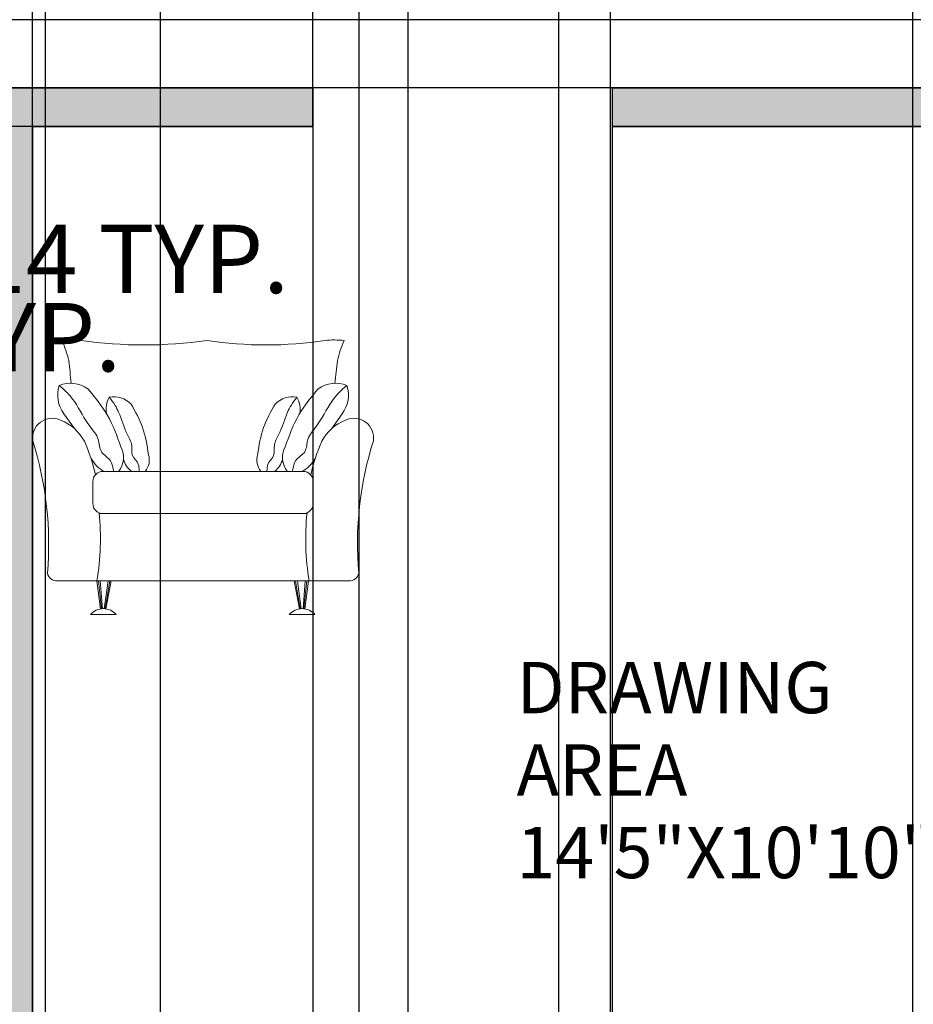
# Model space of a CAD drawing. Units: inches. Extents: x -24 to 368, y -370 to 58.
# Tile 5 of 9: x 130 to 235, y -255 to -140. Entities that reach past the tile are written whole.
import ezdxf

# ---------------------------------------------------------------- set-up
doc = ezdxf.new("R2010")
doc.units = ezdxf.units.IN
doc.header["$MEASUREMENT"] = 0
for name, color, linetype, lineweight in [('A-ANNO-DIMS', 2, 'Continuous', 18), ('A-AREA-IDEN', 7, 'Continuous', 18), ('A-WALL', 7, 'Continuous', 35), ('Furniture', 7, 'Continuous', 15)]:
    doc.layers.add(name, color=color, linetype=linetype, lineweight=lineweight)
doc.layers.add('A-DOOR', color=40, linetype='Continuous', lineweight=25, true_color=0xf8d731)
doc.layers.add('A-WALL-PATT', color=18, linetype='Continuous', lineweight=13, true_color=0x000000)
doc.styles.get("Standard").update_dxf_attribs({"font": 'arial.ttf'})
doc.dimstyles.get("Standard").update_dxf_attribs({"dimtxt": 8, "dimasz": 0.18, "dimexe": 0.18, "dimexo": 0.0625, "dimgap": 0.09, "dimtad": 0, "dimtih": 1, "dimtoh": 1, "dimdec": 4, "dimzin": 0, "dimdsep": 46, "dimlunit": 3, "dimtxsty": 'Standard', "dimcen": 0.09, "dimclre": 5, "dimclrt": 6, "dimadec": 0, "dimazin": 0, "dimtfac": 1, "dimtdec": 4, "dimtofl": 0, "dimtmove": 0, "dimatfit": 3, "dimfxl": 1, "dimtolj": 1, "dimtzin": 0, "dimarcsym": 0})

# ---------------------------------------------------------------- blocks, each defined once
blk = doc.blocks.new('*D11')
at = {"layer": 'A-ANNO-DIMS', "color": 5, "lineweight": -2, "transparency": 16777216}
for p, q in [((104.31, -160.81), (106.54, -160.81)), ((104.31, -174.87), (106.54, -174.87))]:
    blk.add_line(p, q, dxfattribs=at)
at = {"layer": 'A-ANNO-DIMS', "color": 0, "lineweight": -2, "transparency": 16777216}
for p, q in [((106.36, -160.99), (106.36, -163.61)), ((106.36, -174.69), (106.36, -172.07))]:
    blk.add_line(p, q, dxfattribs=at)
at = {"layer": 'A-ANNO-DIMS', "color": 0, "transparency": 16777216}
for points in [[(106.33, -160.99), (106.39, -160.99), (106.36, -160.81)], [(106.33, -174.69), (106.39, -174.69), (106.36, -174.87)]]:
    blk.add_solid(points, dxfattribs=at)
at = {"layer": 'Defpoints', "color": 0, "transparency": 16777216}
for p in [(104.24, -160.81), (106.36, -160.81), (104.24, -174.87)]:
    blk.add_point(p, dxfattribs=at)
at = {"layer": 'A-ANNO-DIMS', "color": 6, "transparency": 16777216, "insert": (106.36, -167.84), "char_height": 8, "attachment_point": 5}
blk.add_mtext('\\A1;DINING CHAIR 14 TYP.', dxfattribs=at)
blk = doc.blocks.new('*D12')
at = {"layer": 'A-ANNO-DIMS', "color": 5, "lineweight": -2, "transparency": 16777216}
for p, q in [((90.76, -174.94), (90.76, -177.17)), ((104.24, -174.94), (104.24, -177.17))]:
    blk.add_line(p, q, dxfattribs=at)
at = {"layer": 'A-ANNO-DIMS', "color": 0, "lineweight": -2, "transparency": 16777216}
for p, q in [((90.94, -176.99), (104.06, -176.99)), ((104.24, -176.99), (104.42, -176.99))]:
    blk.add_line(p, q, dxfattribs=at)
at = {"layer": 'A-ANNO-DIMS', "color": 0, "transparency": 16777216}
for points in [[(90.94, -176.96), (90.94, -177.02), (90.76, -176.99)], [(104.06, -176.96), (104.06, -177.02), (104.24, -176.99)]]:
    blk.add_solid(points, dxfattribs=at)
at = {"layer": 'Defpoints', "color": 0, "transparency": 16777216}
for p in [(90.76, -174.87), (104.24, -174.87), (104.24, -176.99)]:
    blk.add_point(p, dxfattribs=at)
at = {"layer": 'A-ANNO-DIMS', "color": 6, "transparency": 16777216, "insert": (123.61, -176.99), "char_height": 8, "attachment_point": 5}
blk.add_mtext('\\A1;13 TYP.', dxfattribs=at)
blk = doc.blocks.new('*D42')
at = {"layer": 'A-ANNO-DIMS', "color": 5, "lineweight": -2, "transparency": 16777216}
for p, q in [((169.81, 24.59), (169.81, -363.55)), ((193.16, 24.58), (193.16, -363.55))]:
    blk.add_line(p, q, dxfattribs=at)
at = {"layer": 'A-ANNO-DIMS', "color": 0, "lineweight": -2, "transparency": 16777216}
for p, q in [((169.99, -363.37), (192.98, -363.37)), ((193.16, -363.37), (193.34, -363.37))]:
    blk.add_line(p, q, dxfattribs=at)
at = {"layer": 'A-ANNO-DIMS', "color": 0, "transparency": 16777216}
for points in [[(169.99, -363.34), (169.99, -363.4), (169.81, -363.37)], [(192.98, -363.34), (192.98, -363.4), (193.16, -363.37)]]:
    blk.add_solid(points, dxfattribs=at)
at = {"layer": 'Defpoints', "color": 0, "transparency": 16777216}
for p in [(169.81, 24.65), (193.16, 24.64), (193.16, -363.37)]:
    blk.add_point(p, dxfattribs=at)
at = {"layer": 'A-ANNO-DIMS', "color": 6, "transparency": 16777216, "insert": (207.03, -363.37), "char_height": 8, "attachment_point": 5}
blk.add_mtext('\\A1;23.35', dxfattribs=at)
blk = doc.blocks.new('*D51')
at = {"layer": 'A-ANNO-DIMS', "color": 5, "lineweight": -2, "transparency": 16777216}
for p, q in [((175.57, -303.29), (175.57, 52.85)), ((234.57, -303.29), (234.57, 52.85))]:
    blk.add_line(p, q, dxfattribs=at)
at = {"layer": 'A-ANNO-DIMS', "color": 0, "lineweight": -2, "transparency": 16777216}
for p, q in [((175.75, 52.67), (199.24, 52.67)), ((234.39, 52.67), (210.9, 52.67))]:
    blk.add_line(p, q, dxfattribs=at)
at = {"layer": 'A-ANNO-DIMS', "color": 0, "transparency": 16777216}
for points in [[(175.75, 52.7), (175.75, 52.64), (175.57, 52.67)], [(234.39, 52.7), (234.39, 52.64), (234.57, 52.67)]]:
    blk.add_solid(points, dxfattribs=at)
at = {"layer": 'Defpoints', "color": 0, "transparency": 16777216}
for p in [(234.57, 52.67), (175.57, -303.36), (234.57, -303.36)]:
    blk.add_point(p, dxfattribs=at)
at = {"layer": 'A-ANNO-DIMS', "color": 6, "transparency": 16777216, "insert": (205.07, 52.67), "char_height": 8, "attachment_point": 5}
blk.add_mtext('\\A1;59', dxfattribs=at)
blk = doc.blocks.new('*D55')
at = {"layer": 'A-ANNO-DIMS', "color": 5, "lineweight": -2, "transparency": 16777216}
for p, q in [((131.66, -152.29), (131.66, 52.85)), ((164.43, -152.29), (164.43, 52.85))]:
    blk.add_line(p, q, dxfattribs=at)
at = {"layer": 'A-ANNO-DIMS', "color": 0, "lineweight": -2, "transparency": 16777216}
for p, q in [((131.84, 52.67), (134.46, 52.67)), ((164.25, 52.67), (161.63, 52.67))]:
    blk.add_line(p, q, dxfattribs=at)
at = {"layer": 'A-ANNO-DIMS', "color": 0, "transparency": 16777216}
for points in [[(131.84, 52.7), (131.84, 52.64), (131.66, 52.67)], [(164.25, 52.7), (164.25, 52.64), (164.43, 52.67)]]:
    blk.add_solid(points, dxfattribs=at)
at = {"layer": 'Defpoints', "color": 0, "transparency": 16777216}
for p in [(164.43, 52.67), (131.66, -152.36), (164.43, -152.36)]:
    blk.add_point(p, dxfattribs=at)
at = {"layer": 'A-ANNO-DIMS', "color": 6, "transparency": 16777216, "insert": (148.05, 52.67), "char_height": 8, "attachment_point": 5}
blk.add_mtext('\\A1;32.77', dxfattribs=at)
blk = doc.blocks.new('*D56')
at = {"layer": 'A-ANNO-DIMS', "color": 5, "lineweight": -2, "transparency": 16777216}
for p, q in [((164.43, -152.42), (164.43, -363.55)), ((199.43, -152.42), (199.43, -363.55))]:
    blk.add_line(p, q, dxfattribs=at)
at = {"layer": 'A-ANNO-DIMS', "color": 0, "lineweight": -2, "transparency": 16777216}
for p, q in [((164.61, -363.37), (176.08, -363.37)), ((199.25, -363.37), (187.78, -363.37))]:
    blk.add_line(p, q, dxfattribs=at)
at = {"layer": 'A-ANNO-DIMS', "color": 0, "transparency": 16777216}
for points in [[(164.61, -363.34), (164.61, -363.4), (164.43, -363.37)], [(199.25, -363.34), (199.25, -363.4), (199.43, -363.37)]]:
    blk.add_solid(points, dxfattribs=at)
at = {"layer": 'Defpoints', "color": 0, "transparency": 16777216}
for p in [(164.43, -152.36), (199.43, -152.36), (199.43, -363.37)]:
    blk.add_point(p, dxfattribs=at)
at = {"layer": 'A-ANNO-DIMS', "color": 6, "transparency": 16777216, "insert": (181.93, -363.37), "char_height": 8, "attachment_point": 5}
blk.add_mtext('\\A1;35', dxfattribs=at)
blk = doc.blocks.new('*D57')
at = {"layer": 'A-ANNO-DIMS', "color": 5, "lineweight": -2, "transparency": 16777216}
for p, q in [((164.37, -147.86), (-15.03, -147.86)), ((164.37, -152.36), (-15.03, -152.36))]:
    blk.add_line(p, q, dxfattribs=at)
at = {"layer": 'A-ANNO-DIMS', "color": 0, "lineweight": -2, "transparency": 16777216}
for p, q in [((-14.85, -147.86), (-14.85, -147.68)), ((-14.85, -147.68), (-14.67, -147.68)), ((-14.85, -152.18), (-14.85, -148.04))]:
    blk.add_line(p, q, dxfattribs=at)
at = {"layer": 'A-ANNO-DIMS', "color": 0, "transparency": 16777216}
for points in [[(-14.88, -148.04), (-14.82, -148.04), (-14.85, -147.86)], [(-14.88, -152.18), (-14.82, -152.18), (-14.85, -152.36)]]:
    blk.add_solid(points, dxfattribs=at)
at = {"layer": 'Defpoints', "color": 0, "transparency": 16777216}
for p in [(-14.85, -147.86), (164.43, -147.86), (164.43, -152.36)]:
    blk.add_point(p, dxfattribs=at)
at = {"layer": 'A-ANNO-DIMS', "color": 6, "transparency": 16777216, "insert": (-7.11, -147.68), "char_height": 8, "attachment_point": 5}
blk.add_mtext('\\A1;4.5', dxfattribs=at)
blk = doc.blocks.new('*D58')
at = {"layer": 'A-ANNO-DIMS', "color": 5, "lineweight": -2, "transparency": 16777216}
for p, q in [((133.16, -31.92), (133.16, -363.55)), ((146.57, -31.92), (146.57, -363.55))]:
    blk.add_line(p, q, dxfattribs=at)
at = {"layer": 'A-ANNO-DIMS', "color": 0, "lineweight": -2, "transparency": 16777216}
for p, q in [((133.34, -363.37), (146.39, -363.37)), ((146.57, -363.37), (146.75, -363.37))]:
    blk.add_line(p, q, dxfattribs=at)
at = {"layer": 'A-ANNO-DIMS', "color": 0, "transparency": 16777216}
for points in [[(133.34, -363.34), (133.34, -363.4), (133.16, -363.37)], [(146.39, -363.34), (146.39, -363.4), (146.57, -363.37)]]:
    blk.add_solid(points, dxfattribs=at)
at = {"layer": 'Defpoints', "color": 0, "transparency": 16777216}
for p in [(133.16, -31.86), (146.57, -31.86), (146.57, -363.37)]:
    blk.add_point(p, dxfattribs=at)
at = {"layer": 'A-ANNO-DIMS', "color": 6, "transparency": 16777216, "insert": (163.1, -363.37), "char_height": 8, "attachment_point": 5}
blk.add_mtext('\\A1;13.405', dxfattribs=at)
blk = doc.blocks.new('*D59')
at = {"layer": 'A-ANNO-DIMS', "color": 5, "lineweight": -2, "transparency": 16777216}
for p, q in [((246.6, -139.91), (-15.03, -139.91)), ((246.6, -147.86), (-15.03, -147.86))]:
    blk.add_line(p, q, dxfattribs=at)
at = {"layer": 'A-ANNO-DIMS', "color": 0, "lineweight": -2, "transparency": 16777216}
for p, q in [((-14.85, -139.91), (-14.85, -139.73)), ((-14.85, -139.73), (-14.67, -139.73)), ((-14.85, -147.68), (-14.85, -140.09))]:
    blk.add_line(p, q, dxfattribs=at)
at = {"layer": 'A-ANNO-DIMS', "color": 0, "transparency": 16777216}
for points in [[(-14.88, -140.09), (-14.82, -140.09), (-14.85, -139.91)], [(-14.88, -147.68), (-14.82, -147.68), (-14.85, -147.86)]]:
    blk.add_solid(points, dxfattribs=at)
at = {"layer": 'Defpoints', "color": 0, "transparency": 16777216}
for p in [(-14.85, -139.91), (246.66, -139.91), (246.66, -147.86)]:
    blk.add_point(p, dxfattribs=at)
at = {"layer": 'A-ANNO-DIMS', "color": 6, "transparency": 16777216, "insert": (-4.2, -139.73), "char_height": 8, "attachment_point": 5}
blk.add_mtext('\\A1;7.95', dxfattribs=at)
blk = doc.blocks.new('*D60')
at = {"layer": 'A-ANNO-DIMS', "color": 5, "lineweight": -2, "transparency": 16777216}
for p, q in [((133.16, -93.92), (133.16, -363.55)), ((193.16, -95.92), (193.16, -363.55))]:
    blk.add_line(p, q, dxfattribs=at)
at = {"layer": 'A-ANNO-DIMS', "color": 0, "lineweight": -2, "transparency": 16777216}
for p, q in [((133.34, -363.37), (157.33, -363.37)), ((192.98, -363.37), (168.99, -363.37))]:
    blk.add_line(p, q, dxfattribs=at)
at = {"layer": 'A-ANNO-DIMS', "color": 0, "transparency": 16777216}
for points in [[(133.34, -363.34), (133.34, -363.4), (133.16, -363.37)], [(192.98, -363.34), (192.98, -363.4), (193.16, -363.37)]]:
    blk.add_solid(points, dxfattribs=at)
at = {"layer": 'Defpoints', "color": 0, "transparency": 16777216}
for p in [(133.16, -93.86), (193.16, -95.86), (193.16, -363.37)]:
    blk.add_point(p, dxfattribs=at)
at = {"layer": 'A-ANNO-DIMS', "color": 6, "transparency": 16777216, "insert": (163.16, -363.37), "char_height": 8, "attachment_point": 5}
blk.add_mtext('\\A1;60', dxfattribs=at)
blk = doc.blocks.new('*D65')
at = {"layer": 'A-ANNO-DIMS', "color": 5, "lineweight": -2, "transparency": 16777216}
for p, q in [((105.95, -335.29), (105.95, 52.85)), ((127.16, -335.29), (127.16, 52.85))]:
    blk.add_line(p, q, dxfattribs=at)
at = {"layer": 'A-ANNO-DIMS', "color": 0, "lineweight": -2, "transparency": 16777216}
for p, q in [((106.13, 52.67), (126.98, 52.67)), ((127.16, 52.67), (127.34, 52.67))]:
    blk.add_line(p, q, dxfattribs=at)
at = {"layer": 'A-ANNO-DIMS', "color": 0, "transparency": 16777216}
for points in [[(106.13, 52.7), (106.13, 52.64), (105.95, 52.67)], [(126.98, 52.7), (126.98, 52.64), (127.16, 52.67)]]:
    blk.add_solid(points, dxfattribs=at)
at = {"layer": 'Defpoints', "color": 0, "transparency": 16777216}
for p in [(127.16, 52.67), (105.95, -335.36), (127.16, -335.36)]:
    blk.add_point(p, dxfattribs=at)
at = {"layer": 'A-ANNO-DIMS', "color": 6, "transparency": 16777216, "insert": (140.23, 52.67), "char_height": 8, "attachment_point": 5}
blk.add_mtext('\\A1;21.21', dxfattribs=at)
blk = doc.blocks.new('*D70')
at = {"layer": 'A-ANNO-DIMS', "color": 5, "lineweight": -2, "transparency": 16777216}
for p, q in [((193.16, -95.92), (193.16, -363.55)), ((199.21, -95.92), (199.21, -363.55))]:
    blk.add_line(p, q, dxfattribs=at)
at = {"layer": 'A-ANNO-DIMS', "color": 0, "lineweight": -2, "transparency": 16777216}
for p, q in [((193.34, -363.37), (199.03, -363.37)), ((199.21, -363.37), (199.39, -363.37))]:
    blk.add_line(p, q, dxfattribs=at)
at = {"layer": 'A-ANNO-DIMS', "color": 0, "transparency": 16777216}
for points in [[(193.34, -363.34), (193.34, -363.4), (193.16, -363.37)], [(199.03, -363.34), (199.03, -363.4), (199.21, -363.37)]]:
    blk.add_solid(points, dxfattribs=at)
at = {"layer": 'Defpoints', "color": 0, "transparency": 16777216}
for p in [(193.16, -95.86), (199.21, -95.86), (199.21, -363.37)]:
    blk.add_point(p, dxfattribs=at)
at = {"layer": 'A-ANNO-DIMS', "color": 6, "transparency": 16777216, "insert": (212.23, -363.37), "char_height": 8, "attachment_point": 5}
blk.add_mtext('\\A1;6.051', dxfattribs=at)

msp = doc.modelspace()

# ---------------------------------------------------------------- hatches: boundary and pattern name
at = {"layer": 'A-WALL-PATT'}
h = msp.add_hatch(color=256, dxfattribs=at)
h.dxf.hatch_style = 1
h.paths.add_polyline_path([(13.1621, -93.8573), (80.4499, -93.8573), (80.4499, -89.3573), (13.1621, -89.3573), (13.1621, -61.0987), (4.1621, -61.0987), (4.1621, -149.8573), (13.1621, -149.8573)])
h.paths.add_polyline_path([(146.5668, -27.3573), (133.1621, -27.3573), (133.1621, 10.3323), (133.1272, 10.3313), (133.1621, 24.6427), (139.8141, 24.6427), (139.8141, 33.6427), (95.3329, 33.6427), (95.3329, 24.6427), (128.6621, 24.6427), (128.6621, -89.3573), (127.4499, -89.3573), (127.4499, -93.8573), (133.1621, -93.8573), (133.1621, -31.8573), (146.5668, -31.8573)])
h.paths.add_polyline_path([(197.6621, 24.6427), (236.2134, 24.6427), (236.2134, 33.6427), (169.8141, 33.6427), (169.8141, 24.6427), (193.1621, 24.6427), (193.1621, -27.3573), (181.5668, -27.3573), (181.5668, -31.8573), (193.1621, -31.8573), (193.1621, -95.8573), (199.2127, -95.8573), (199.2127, -91.3573), (197.6621, -91.3573)])
h.paths.add_polyline_path([(322.1621, -52.531), (313.1621, -52.531), (313.1621, -91.3573), (246.2127, -91.3573), (246.2127, -95.8573), (246.6621, -95.8573), (246.6621, -104.9077), (251.1621, -104.9077), (251.1621, -95.8573), (313.1621, -95.8573), (313.1621, -105.6922), (317.6621, -105.6922), (322.1621, -105.6922)])
h.paths.add_polyline_path([(322.1621, -135.6922), (313.1621, -135.6922), (313.1621, -147.8573), (251.1621, -147.8573), (251.1621, -139.9077), (246.6621, -139.9077), (246.6621, -147.8573), (199.43, -147.8573), (199.43, -152.3573), (313.1621, -152.3573), (313.1621, -194.6142), (317.6621, -194.6142), (322.1621, -194.6142)])
h.paths.add_polyline_path([(322.1621, -241.6142), (313.1621, -241.6142), (313.1621, -275.3573), (287.3912, -275.3573), (287.3912, -279.8573), (313.1621, -279.8573), (313.1621, -335.3573), (298.077, -335.3573), (298.077, -344.3573), (322.1621, -344.3573)])
h.paths.add_polyline_path([(263.077, -335.3573), (241.1621, -335.3573), (241.1621, -279.8573), (252.3912, -279.8573), (252.3912, -275.3573), (236.6621, -275.3573), (236.6621, -298.8573), (234.5689, -298.8573), (234.5689, -303.3573), (236.6621, -303.3573), (236.6621, -344.3573), (263.077, -344.3573), (263.077, -339.8573)])
h.paths.add_polyline_path([(175.5689, -298.8573), (131.6621, -298.8573), (131.6621, -152.3573), (164.43, -152.3573), (164.43, -147.8573), (127.1621, -147.8573), (127.1621, -232.8573), (117.1621, -232.8573), (117.1621, -237.3573), (127.1621, -237.3573), (127.1621, -335.3573), (84.4055, -335.3573), (84.4055, -344.3573), (131.6621, -344.3573), (131.6621, -303.3573), (175.5689, -303.3573)])
h.paths.add_polyline_path([(70.1621, -232.8573), (13.1621, -232.8573), (13.1621, -196.8573), (4.1621, -196.8573), (4.1621, -257.9061), (13.1621, -257.9061), (13.1621, -237.3573), (70.1621, -237.3573)])
h.paths.add_polyline_path([(13.1621, -304.9061), (4.1621, -304.9061), (4.1621, -344.3573), (37.4055, -344.3573), (37.4055, -335.3573), (13.1621, -335.3573)])
h.paths.add_polyline_path([(322.1621, 33.6427), (283.2134, 33.6427), (283.2134, 24.6427), (313.1621, 24.6427), (313.1621, 11.9273), (313.4656, 11.629), (313.1621, 11.629), (313.1621, -5.531), (322.1621, -5.531)])
h.paths.add_polyline_path([(48.3329, 33.6427), (4.1621, 33.6427), (4.1621, -14.0987), (13.1621, -14.0987), (13.1621, 24.6427), (48.3329, 24.6427)])

# ---------------------------------------------------------------- linework, layer by layer
at = {"layer": 'A-DOOR'}
for p, q in [((164.43, -147.8573), (164.43, -152.3573)), ((199.43, -147.8573), (199.43, -152.3573))]:
    msp.add_line(p, q, dxfattribs=at)
at = {"layer": 'A-WALL'}
for p, q in [((127.1621, -147.8573), (164.43, -147.8573)), ((199.43, -147.8573), (246.6621, -147.8573)), ((131.6621, -298.8573), (131.6621, -152.3573)), ((131.6621, -152.3573), (164.43, -152.3573)), ((199.43, -152.3573), (313.1621, -152.3573))]:
    msp.add_line(p, q, dxfattribs=at)
at = {"layer": 'Furniture'}
for p, q in [((135.3283, -185.9394), (136.5534, -187.6639)), ((167.8727, -185.9394), (166.6476, -187.6639)), ((139.8967, -192.6699), (156.291, -192.6699)), ((153.2449, -192.6699), (163.3043, -192.6699)), ((138.7156, -193.851), (138.7156, -196.4214)), ((164.4854, -193.851), (164.4854, -196.4214)), ((139.4445, -197.6025), (159.5867, -197.6025)), ((153.2449, -197.6025), (163.7565, -197.6025)), ((134.547, -205.4765), (168.6539, -205.4765)), ((139.1919, -205.4765), (139.6068, -208.7552)), ((139.3883, -205.4765), (139.7331, -208.7356)), ((139.5778, -205.4765), (139.8249, -208.7249)), ((140.4996, -205.4765), (140.0386, -208.7239)), ((140.7011, -205.4765), (140.1691, -208.7395)), ((140.8729, -205.4765), (140.2331, -208.7494)), ((162.2515, -205.4765), (162.8913, -208.7494)), ((162.4233, -205.4765), (162.9553, -208.7395)), ((162.6248, -205.4765), (163.0857, -208.7239)), ((163.5466, -205.4765), (163.2995, -208.7249)), ((163.7361, -205.4765), (163.3913, -208.7356)), ((163.9325, -205.4765), (163.5176, -208.7552)), ((138.4424, -209.4135), (141.4422, -209.4135)), ((164.682, -209.4135), (161.6822, -209.4135))]:
    msp.add_line(p, q, dxfattribs=at)
for centre, radius, start, end in [((136.2882, -187.7508), 10.4394, 84.309433, 96.53714), ((124.4097, -182.3319), 11.7815, 12.865036, 24.858118), ((144.6849, -126.7059), 51.1891, 261.731512, 278.28801), ((158.9788, -132.9067), 44.9883, 261.158178, 278.82099), ((166.9128, -187.7508), 10.4394, 83.46286, 95.690567), ((178.7912, -182.3319), 11.7815, 155.141882, 167.134964), ((-33.5561, -199.5273), 170.6066, 5.76863, 6.670835), ((336.7571, -199.5273), 170.6066, 173.329165, 174.23137), ((138.2353, -183.764), 3.6309, 161.668804, 216.808795), ((136.0859, -185.9472), 3.5693, 55.070624, 111.311814), ((167.1151, -185.9472), 3.5693, 68.688186, 124.929376), ((164.9656, -183.764), 3.6309, 323.191205, 18.331196), ((143.1599, -185.4079), 2.9047, 151.007865, 189.441488), ((141.1469, -186.8063), 2.8555, 44.409684, 100.650875), ((162.054, -186.8063), 2.8555, 79.349125, 135.590316), ((160.0411, -185.4079), 2.9047, 350.558512, 28.992135), ((133.9851, -188.7798), 2.323, 65.372265, 188.220886), ((132.8939, -191.7614), 5.4938, 28.477957, 67.987132), ((170.307, -191.7614), 5.4938, 112.012868, 151.522043), ((169.2159, -188.7798), 2.323, 351.779114, 114.627735), ((94.0394, -201.1117), 39.5128, 354.968953, 17.679552), ((119.7255, -197.2093), 19.7229, 12.110834, 24.14463), ((139.7067, -191.0309), 2.6003, 320.925151, 27.981764), ((163.4942, -191.0309), 2.6003, 152.018236, 219.074849), ((183.4754, -197.2093), 19.7229, 155.85537, 167.889166), ((209.1616, -201.1117), 39.5128, 162.320448, 185.031047), ((143.2412, -191.3389), 2.0802, 320.219216, 17.320825), ((159.9597, -191.3389), 2.0802, 162.679175, 219.780784), ((141.7408, -189.4826), 3.6309, 207.873103, 241.381252), ((145.0695, -190.4227), 2.9047, 197.212164, 230.720312), ((158.1315, -190.4227), 2.9047, 309.279688, 342.787836), ((161.4602, -189.4826), 3.6309, 298.618748, 332.126897), ((139.8967, -193.851), 1.1811, 90, 180), ((163.3043, -193.851), 1.1811, 0, 90), ((139.8967, -196.4214), 1.1811, 180, 270), ((163.3043, -196.4214), 1.1811, 270, 0), ((109.9786, -200.5586), 29.6244, 350.444113, 5.900441), ((193.2224, -200.5586), 29.6244, 174.099559, 189.555887), ((134.547, -204.2954), 1.1811, 193.782782, 270), ((168.6539, -204.2954), 1.1811, 270, 346.217218), ((139.9423, -210.6604), 1.9505, 39.737069, 140.262931), ((163.1821, -210.6604), 1.9505, 39.737069, 140.262931)]:
    msp.add_arc(centre, radius, start, end, dxfattribs=at)
for points, knots in [([(134.7886, -182.622), (135.1615, -182.9453), (135.8153, -183.5123), (137.0489, -185.1218), (137.9235, -187.0454), (139.5156, -188.7407), (139.4361, -190.5405), (140.885, -191.1903), (141.0244, -192.1648), (141.1396, -192.5795), (141.1665, -192.6699)], [0, 0, 0, 0, 37.5062875, 65.78225886, 153.61965792, 198.46528521, 236.49588263, 274.83716127, 300.24284214, 307.42837957, 307.42837957, 307.42837957, 307.42837957]), ([(168.4123, -182.622), (168.0395, -182.9453), (167.3856, -183.5123), (166.1521, -185.1218), (165.2775, -187.0454), (163.6854, -188.7407), (163.7649, -190.5405), (162.316, -191.1903), (162.1765, -192.1648), (162.0614, -192.5795), (162.0345, -192.6699)], [0, 0, 0, 0, 37.5062875, 65.78225886, 153.61965792, 198.46528521, 236.49588263, 274.83716127, 300.24284214, 307.42837957, 307.42837957, 307.42837957, 307.42837957]), ([(138.1296, -183.0209), (138.9508, -184.0011), (140.6503, -186.0294), (141.5422, -188.5226), (142.003, -189.8109)], [0, 0, 0, 0, 3.80449985, 7.87243062, 7.87243062, 7.87243062, 7.87243062]), ([(140.6191, -184), (140.8644, -184.3094), (141.2946, -184.8519), (142.0262, -186.2999), (142.4291, -187.9416), (143.4299, -189.5101), (143.101, -190.9133), (144.144, -191.6386), (144.112, -192.3643), (144.13, -192.6521), (144.1312, -192.6699)], [0, 0, 0, 0, 37.5062875, 65.78225886, 153.61965792, 198.46528521, 236.49588263, 274.83716127, 300.24284214, 301.92697141, 301.92697141, 301.92697141, 301.92697141]), ([(162.5818, -184), (162.3365, -184.3094), (161.9064, -184.8519), (161.1748, -186.2999), (160.7719, -187.9416), (159.7711, -189.5101), (160.1, -190.9133), (159.057, -191.6386), (159.0889, -192.3643), (159.071, -192.6521), (159.0698, -192.6699)], [0, 0, 0, 0, 37.5062875, 65.78225886, 153.61965792, 198.46528521, 236.49588263, 274.83716127, 300.24284214, 301.92697141, 301.92697141, 301.92697141, 301.92697141]), ([(165.0714, -183.0209), (164.2501, -184.0011), (162.5507, -186.0294), (161.6588, -188.5226), (161.1979, -189.8109)], [0, 0, 0, 0, 3.80449985, 7.87243062, 7.87243062, 7.87243062, 7.87243062]), ([(143.1867, -184.8081), (143.6873, -185.7003), (144.7232, -187.5464), (145.0554, -189.6385), (145.2271, -190.7196)], [0, 0, 0, 0, 3.04359988, 6.2979445, 6.2979445, 6.2979445, 6.2979445]), ([(160.0142, -184.8081), (159.5136, -185.7003), (158.4777, -187.5464), (158.1455, -189.6385), (157.9739, -190.7196)], [0, 0, 0, 0, 3.04359988, 6.2979445, 6.2979445, 6.2979445, 6.2979445])]:
    msp.add_open_spline(points, degree=3, knots=knots, dxfattribs=at)

# ---------------------------------------------------------------- texts
at = {"layer": 'A-AREA-IDEN'}
for s, p in [('DRAWING', (188.2434, -220.9324)), ('AREA', (188.2434, -230.5709)), ('14\'5"X10\'10"', (188.2434, -240.2094))]:
    msp.add_text(s, height=6, dxfattribs=at).set_placement(p)

# ---------------------------------------------------------------- dimensions: what is measured, and where the dimension line sits
at = {"layer": 'A-ANNO-DIMS'}
for base, p1, p2, override, picture, middle in [((127.1621, 52.6658), (105.953, -335.3573), (127.1621, -335.3573), {"dimdec": 2, "dimlfac": 1, "dimrnd": 0, "dimzin": 0, "dimdsep": 46, "dimlunit": 2}, '*D65', (140.2261, 52.6658)), ((164.43, 52.6658), (131.6621, -152.3573), (164.43, -152.3573), {"dimdec": 2, "dimlfac": 1, "dimrnd": 0, "dimzin": 0, "dimdsep": 46, "dimlunit": 2}, '*D55', (148.046, 52.6658)), ((234.5689, 52.6658), (175.5689, -303.3573), (234.5689, -303.3573), {"dimdec": 0, "dimlfac": 1, "dimrnd": 0, "dimzin": 0, "dimdsep": 46, "dimlunit": 2}, '*D51', (205.0689, 52.6658)), ((193.1621, -363.3723), (169.8141, 24.6508), (193.1621, 24.6427), {"dimdec": 2, "dimlfac": 1, "dimrnd": 0, "dimzin": 0, "dimdsep": 46, "dimlunit": 2}, '*D42', (207.0283, -363.3723)), ((146.5668, -363.3723), (133.1621, -31.8573), (146.5668, -31.8573), {"dimdec": 3, "dimlfac": 1, "dimrnd": 0, "dimzin": 0, "dimdsep": 46, "dimlunit": 2}, '*D58', (163.096, -363.3723)), ((193.1621, -363.3723), (133.1621, -93.8573), (193.1621, -95.8573), {"dimdec": 0, "dimlfac": 1, "dimrnd": 0, "dimzin": 0, "dimdsep": 46, "dimlunit": 2}, '*D60', (163.1621, -363.3723)), ((199.2127, -363.3723), (193.1621, -95.8573), (199.2127, -95.8573), {"dimdec": 3, "dimlfac": 1, "dimrnd": 0, "dimzin": 0, "dimdsep": 46, "dimlunit": 2}, '*D70', (212.2304, -363.3723)), ((199.43, -363.3723), (164.43, -152.3573), (199.43, -152.3573), {"dimdec": 0, "dimlfac": 1, "dimrnd": 0, "dimzin": 0, "dimdsep": 46, "dimlunit": 2}, '*D56', (181.93, -363.3723))]:
    dim = msp.add_linear_dim(base=base, p1=p1, p2=p2, dimstyle='Standard', override=override, dxfattribs=at)
    dim.commit()
    dim.dimension.update_dxf_attribs({"geometry": picture, "text_midpoint": middle})
for base, p1, p2, override, picture, middle in [((-14.8529, -139.9077), (246.6621, -147.8573), (246.6621, -139.9077), {"dimdec": 2, "dimlfac": 1, "dimrnd": 0, "dimzin": 0, "dimdsep": 46, "dimlunit": 2}, '*D59', (-4.1955, -139.7277)), ((-14.8529, -147.8573), (164.43, -152.3573), (164.43, -147.8573), {"dimdec": 1, "dimlfac": 1, "dimrnd": 0, "dimzin": 0, "dimdsep": 46, "dimlunit": 2}, '*D57', (-7.1095, -147.6773))]:
    dim = msp.add_linear_dim(base=base, p1=p1, p2=p2, angle=90, dimstyle='Standard', override=override, dxfattribs=at)
    dim.commit()
    dim.dimension.update_dxf_attribs({"geometry": picture, "text_midpoint": middle})
dim = msp.add_linear_dim(base=(106.3552, -160.806), p1=(104.2448, -174.8749), p2=(104.2448, -160.806), angle=90, text='DINING CHAIR <> TYP.', dimstyle='Standard', override={"dimdec": 0, "dimlfac": 1, "dimrnd": 0, "dimzin": 0, "dimdsep": 46, "dimlunit": 2}, dxfattribs=at)
dim.commit()
dim.dimension.update_dxf_attribs({"geometry": '*D11', "text_midpoint": (106.3552, -167.8404)})
dim = msp.add_linear_dim(base=(104.2448, -176.9852), p1=(90.7557, -174.8749), p2=(104.2448, -174.8749), text='<> TYP.', dimstyle='Standard', override={"dimdec": 0, "dimlfac": 1, "dimrnd": 0, "dimzin": 0, "dimdsep": 46, "dimlunit": 2}, dxfattribs=at)
dim.commit()
dim.dimension.update_dxf_attribs({"geometry": '*D12', "text_midpoint": (123.609, -176.9852)})

doc.saveas('drawing.dxf')
